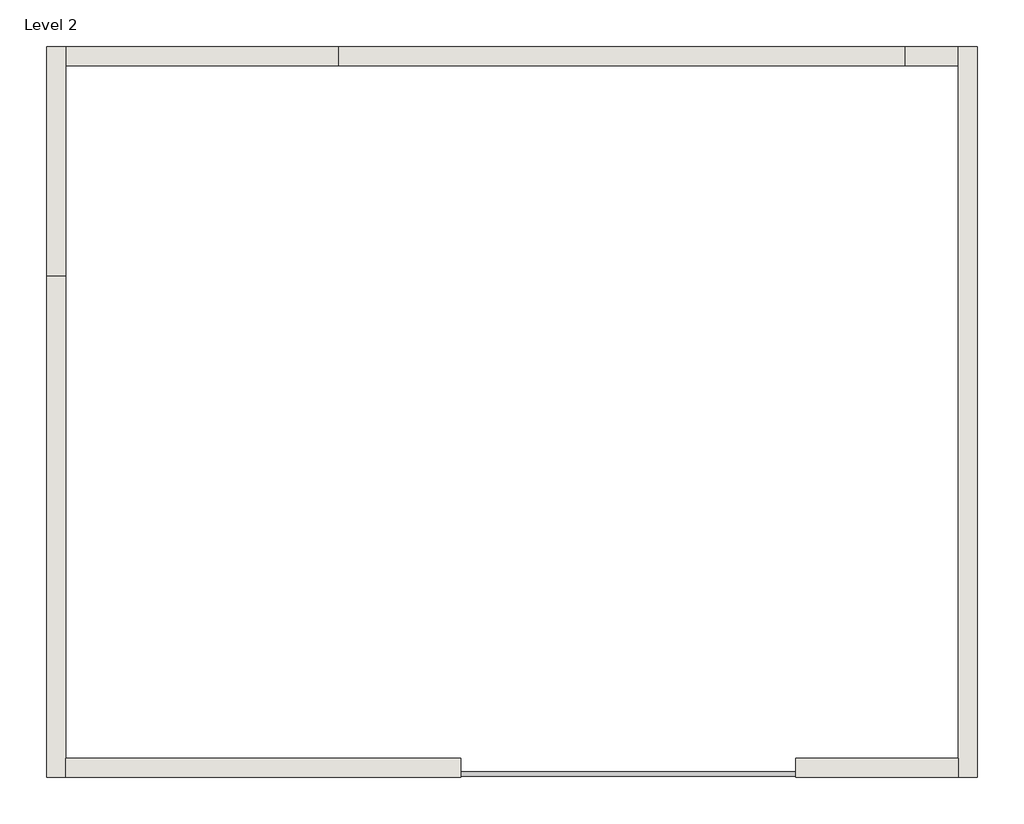
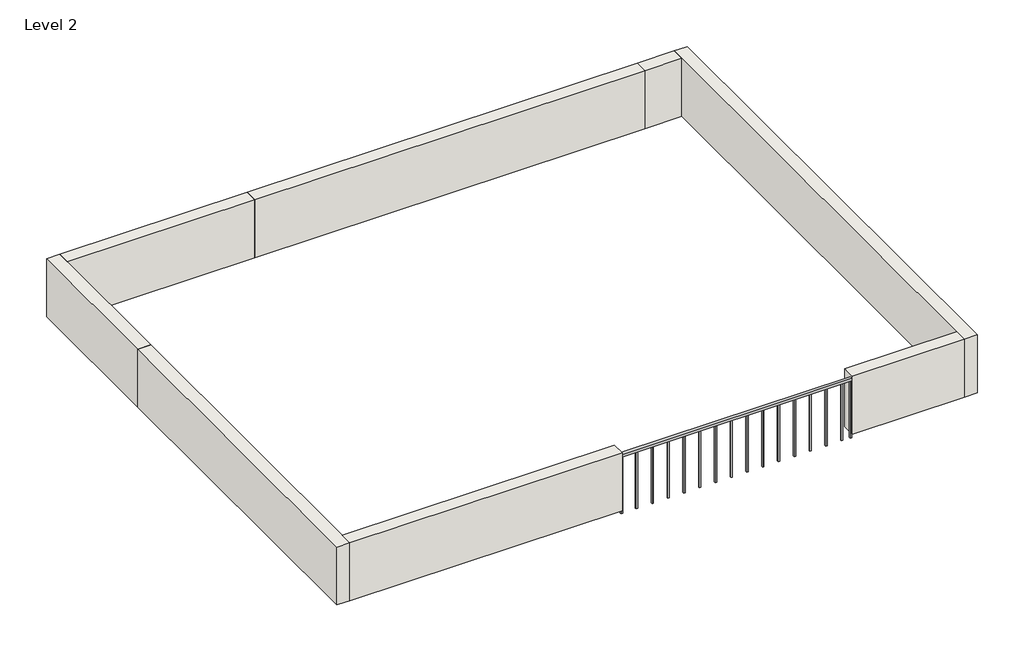
# One storey, incomplete: 8 walls, 1 railing.
"""IFC4 building model written with IfcOpenShell, lengths in millimetres."""

from ifc_helpers import new_model, si_unit, frame, origin, place, context, project, spatial, polyline, outline, extrude, faceted_brep, element, save

model = new_model("IFC4")

# Units and contexts
model_context = context("Model", 3, world=origin())
ifc_project = project(units=[si_unit("LENGTHUNIT", "METRE", prefix="MILLI")], contexts=[model_context])

# Site, building, storey
site = spatial("IfcSite", under=ifc_project)
building = spatial("IfcBuilding", under=site)
storey = spatial("IfcBuildingStorey", under=building, Name="Level 2", Elevation=6400.8)

# Railing
placement = place(None, origin())
element("IfcRailing", 1, ObjectType="1100mm", at=placement, inside=storey, context=model_context, shape_type="SweptSolid", body=[
    extrude(outline(polyline([(-6206.3207599, -3641.6796054), (-6206.3207599, -3591.6796054), (-2193.1207599, -3591.6796054), (-2193.1207599, -3641.6796054), (-6206.3207599, -3641.6796054)])), frame((0.0, 0.0, 7450.8), z_axis=(0.0, 0.0, 1.0), x_axis=(1.0, 0.0, 0.0)), (0.0, 0.0, 1.0), 50.0),
    extrude(outline(polyline([(-2368.8207599, -3629.1796054), (-2368.8207599, -3604.1796054), (-2343.8207599, -3604.1796054), (-2343.8207599, -3629.1796054), (-2368.8207599, -3629.1796054)])), frame((0.0, 0.0, 6400.8), z_axis=(0.0, 0.0, 1.0), x_axis=(1.0, 0.0, 0.0)), (0.0, 0.0, 1.0), 1050.0),
    extrude(outline(polyline([(-2643.8207599, -3629.1796054), (-2643.8207599, -3604.1796054), (-2618.8207599, -3604.1796054), (-2618.8207599, -3629.1796054), (-2643.8207599, -3629.1796054)])), frame((0.0, 0.0, 6400.8), z_axis=(0.0, 0.0, 1.0), x_axis=(1.0, 0.0, 0.0)), (0.0, 0.0, 1.0), 1050.0),
    extrude(outline(polyline([(-2918.8207599, -3629.1796054), (-2918.8207599, -3604.1796054), (-2893.8207599, -3604.1796054), (-2893.8207599, -3629.1796054), (-2918.8207599, -3629.1796054)])), frame((0.0, 0.0, 6400.8), z_axis=(0.0, 0.0, 1.0), x_axis=(1.0, 0.0, 0.0)), (0.0, 0.0, 1.0), 1050.0),
    extrude(outline(polyline([(-3193.8207599, -3629.1796054), (-3193.8207599, -3604.1796054), (-3168.8207599, -3604.1796054), (-3168.8207599, -3629.1796054), (-3193.8207599, -3629.1796054)])), frame((0.0, 0.0, 6400.8), z_axis=(0.0, 0.0, 1.0), x_axis=(1.0, 0.0, 0.0)), (0.0, 0.0, 1.0), 1050.0),
    extrude(outline(polyline([(-3468.8207599, -3629.1796054), (-3468.8207599, -3604.1796054), (-3443.8207599, -3604.1796054), (-3443.8207599, -3629.1796054), (-3468.8207599, -3629.1796054)])), frame((0.0, 0.0, 6400.8), z_axis=(0.0, 0.0, 1.0), x_axis=(1.0, 0.0, 0.0)), (0.0, 0.0, 1.0), 1050.0),
    extrude(outline(polyline([(-3743.8207599, -3629.1796054), (-3743.8207599, -3604.1796054), (-3718.8207599, -3604.1796054), (-3718.8207599, -3629.1796054), (-3743.8207599, -3629.1796054)])), frame((0.0, 0.0, 6400.8), z_axis=(0.0, 0.0, 1.0), x_axis=(1.0, 0.0, 0.0)), (0.0, 0.0, 1.0), 1050.0),
    extrude(outline(polyline([(-4018.8207599, -3629.1796054), (-4018.8207599, -3604.1796054), (-3993.8207599, -3604.1796054), (-3993.8207599, -3629.1796054), (-4018.8207599, -3629.1796054)])), frame((0.0, 0.0, 6400.8), z_axis=(0.0, 0.0, 1.0), x_axis=(1.0, 0.0, 0.0)), (0.0, 0.0, 1.0), 1050.0),
    extrude(outline(polyline([(-4293.8207599, -3629.1796054), (-4293.8207599, -3604.1796054), (-4268.8207599, -3604.1796054), (-4268.8207599, -3629.1796054), (-4293.8207599, -3629.1796054)])), frame((0.0, 0.0, 6400.8), z_axis=(0.0, 0.0, 1.0), x_axis=(1.0, 0.0, 0.0)), (0.0, 0.0, 1.0), 1050.0),
    extrude(outline(polyline([(-4568.8207599, -3629.1796054), (-4568.8207599, -3604.1796054), (-4543.8207599, -3604.1796054), (-4543.8207599, -3629.1796054), (-4568.8207599, -3629.1796054)])), frame((0.0, 0.0, 6400.8), z_axis=(0.0, 0.0, 1.0), x_axis=(1.0, 0.0, 0.0)), (0.0, 0.0, 1.0), 1050.0),
    extrude(outline(polyline([(-4843.8207599, -3629.1796054), (-4843.8207599, -3604.1796054), (-4818.8207599, -3604.1796054), (-4818.8207599, -3629.1796054), (-4843.8207599, -3629.1796054)])), frame((0.0, 0.0, 6400.8), z_axis=(0.0, 0.0, 1.0), x_axis=(1.0, 0.0, 0.0)), (0.0, 0.0, 1.0), 1050.0),
    extrude(outline(polyline([(-5118.8207599, -3629.1796054), (-5118.8207599, -3604.1796054), (-5093.8207599, -3604.1796054), (-5093.8207599, -3629.1796054), (-5118.8207599, -3629.1796054)])), frame((0.0, 0.0, 6400.8), z_axis=(0.0, 0.0, 1.0), x_axis=(1.0, 0.0, 0.0)), (0.0, 0.0, 1.0), 1050.0),
    extrude(outline(polyline([(-5393.8207599, -3629.1796054), (-5393.8207599, -3604.1796054), (-5368.8207599, -3604.1796054), (-5368.8207599, -3629.1796054), (-5393.8207599, -3629.1796054)])), frame((0.0, 0.0, 6400.8), z_axis=(0.0, 0.0, 1.0), x_axis=(1.0, 0.0, 0.0)), (0.0, 0.0, 1.0), 1050.0),
    extrude(outline(polyline([(-5668.8207599, -3629.1796054), (-5668.8207599, -3604.1796054), (-5643.8207599, -3604.1796054), (-5643.8207599, -3629.1796054), (-5668.8207599, -3629.1796054)])), frame((0.0, 0.0, 6400.8), z_axis=(0.0, 0.0, 1.0), x_axis=(1.0, 0.0, 0.0)), (0.0, 0.0, 1.0), 1050.0),
    extrude(outline(polyline([(-5943.8207599, -3629.1796054), (-5943.8207599, -3604.1796054), (-5918.8207599, -3604.1796054), (-5918.8207599, -3629.1796054), (-5943.8207599, -3629.1796054)])), frame((0.0, 0.0, 6400.8), z_axis=(0.0, 0.0, 1.0), x_axis=(1.0, 0.0, 0.0)), (0.0, 0.0, 1.0), 1050.0),
    extrude(outline(polyline([(-2218.1207599, -3629.1796054), (-2218.1207599, -3604.1796054), (-2193.1207599, -3604.1796054), (-2193.1207599, -3629.1796054), (-2218.1207599, -3629.1796054)])), frame((0.0, 0.0, 6400.8), z_axis=(0.0, 0.0, 1.0), x_axis=(1.0, 0.0, 0.0)), (0.0, 0.0, 1.0), 1050.0),
    extrude(outline(polyline([(-6206.3207599, -3629.1796054), (-6206.3207599, -3604.1796054), (-6181.3207599, -3604.1796054), (-6181.3207599, -3629.1796054), (-6206.3207599, -3629.1796054)])), frame((0.0, 0.0, 6400.8), z_axis=(0.0, 0.0, 1.0), x_axis=(1.0, 0.0, 0.0)), (0.0, 0.0, 1.0), 1050.0),
])

# Walls
element("IfcWall", 2, ObjectType="9\"", at=placement, inside=storey, context=model_context, shape_type="Brep", body=[
    faceted_brep([(-13.83523, -3654.7796054, 6477.0), (-13.83523, 5101.6327475, 6477.0), (-13.83523, 5105.4926487, 6477.0), (-13.83523, 5105.4926487, 7543.8), (-13.83523, -3654.7796054, 7543.8), (-242.43523, -3654.7796054, 6477.0), (-242.43523, -3654.7796054, 7543.8), (-242.43523, 4876.8926487, 7543.8), (-242.43523, 5105.4926487, 7543.8), (-242.43523, 5105.4926487, 6477.0), (-242.43523, 4876.8926487, 6477.0)], [[[0, 1, 2, 3, 4]], [[5, 6, 7, 8, 9, 10]], [[2, 1, 0, 5, 10, 9]], [[3, 2, 9, 8]], [[4, 3, 8, 7, 6]], [[0, 4, 6, 5]]]),
])
element("IfcWall", 3, ObjectType="9\"", at=placement, inside=storey, context=model_context, shape_type="SweptSolid", body=[
    extrude(outline(polyline([(-883.78523, 5105.4926487), (-242.43523, 5105.4926487), (-242.43523, 4876.8926487), (-883.78523, 4876.8926487), (-883.78523, 5105.4926487)])), frame((0.0, 0.0, 6477.0), z_axis=(0.0, 0.0, 1.0), x_axis=(1.0, 0.0, 0.0)), (0.0, 0.0, 1.0), 1066.8),
])
element("IfcWall", 4, ObjectType="9\"", at=placement, inside=storey, context=model_context, shape_type="SweptSolid", body=[
    extrude(outline(polyline([(-7680.825513, 5105.4926487), (-883.78523, 5105.4926487), (-883.78523, 4876.8926487), (-7680.825513, 4876.8926487), (-7680.825513, 5105.4926487)])), frame((0.0, 0.0, 6477.0), z_axis=(0.0, 0.0, 1.0), x_axis=(1.0, 0.0, 0.0)), (0.0, 0.0, 1.0), 1066.8),
])
element("IfcWall", 5, ObjectType="9\"", at=placement, inside=storey, context=model_context, shape_type="Brep", body=[
    faceted_brep([(-11175.7858712, 5105.4926487, 6477.0), (-11175.7858712, 2353.0673305, 6477.0), (-11175.7858712, 2353.0673305, 7543.8), (-11175.7858712, 5105.4926487, 7543.8), (-10947.1858712, 5105.4926487, 6477.0), (-10947.1858712, 5105.4926487, 7543.8), (-10947.1858712, 4876.8926487, 7543.8), (-10947.1858712, 2353.0673305, 7543.8), (-10947.1858712, 2353.0673305, 6477.0), (-10947.1858712, 4876.8926487, 6477.0)], [[[0, 1, 2, 3]], [[4, 5, 6, 7, 8, 9]], [[1, 0, 4, 9, 8]], [[2, 1, 8, 7]], [[3, 2, 7, 6, 5]], [[0, 3, 5, 4]]]),
])
element("IfcWall", 6, ObjectType="9\"", at=placement, inside=storey, context=model_context, shape_type="SweptSolid", body=[
    extrude(outline(polyline([(-11175.7858712, -3654.7796054), (-11175.7858712, 2353.0673305), (-10947.1858712, 2353.0673305), (-10947.1858712, -3654.7796054), (-11175.7858712, -3654.7796054)])), frame((0.0, 0.0, 6477.0), z_axis=(0.0, 0.0, 1.0), x_axis=(1.0, 0.0, 0.0)), (0.0, 0.0, 1.0), 1066.8),
])
element("IfcWall", 7, ObjectType="9\"", at=placement, inside=storey, context=model_context, shape_type="SweptSolid", body=[
    extrude(outline(polyline([(-10947.1858712, 5105.4926487), (-7680.825513, 5105.4926487), (-7680.825513, 4876.8926487), (-10947.1858712, 4876.8926487), (-10947.1858712, 5105.4926487)])), frame((0.0, 0.0, 6477.0), z_axis=(0.0, 0.0, 1.0), x_axis=(1.0, 0.0, 0.0)), (0.0, 0.0, 1.0), 1066.8),
])
element("IfcWall", 8, ObjectType="9\"", at=placement, inside=storey, context=model_context, shape_type="SweptSolid", body=[
    extrude(outline(polyline([(-6206.3207599, -3654.7796054), (-10947.1858712, -3654.7796054), (-10947.1858712, -3426.1796054), (-6206.3207599, -3426.1796054), (-6206.3207599, -3654.7796054)])), frame((0.0, 0.0, 6477.0), z_axis=(0.0, 0.0, 1.0), x_axis=(1.0, 0.0, 0.0)), (0.0, 0.0, 1.0), 1066.8),
])
element("IfcWall", 9, ObjectType="9\"", at=placement, inside=storey, context=model_context, shape_type="SweptSolid", body=[
    extrude(outline(polyline([(-242.43523, -3654.7796054), (-2193.1207599, -3654.7796054), (-2193.1207599, -3426.1796054), (-242.43523, -3426.1796054), (-242.43523, -3654.7796054)])), frame((0.0, 0.0, 6477.0), z_axis=(0.0, 0.0, 1.0), x_axis=(1.0, 0.0, 0.0)), (0.0, 0.0, 1.0), 1066.8),
])

save(model, "model.ifc")

# Revit data of these elements
# Type "1100mm"
#   built-in parameter 1008612 = 0.019685 (stored number, unit not read)
#   built-in parameter 1008611 = 0.019685 (stored number, unit not read)
#   built-in parameter 1008609 = 0.902231 (stored number, unit not read)
#   built-in parameter 1008604 = 0.19685 (stored number, unit not read)
#   built-in parameter 1008603 = 0.164042 (stored number, unit not read)
#   Railing Height = 3' - 7.30709"
#   built-in parameter 1008630 = 2
#   built-in parameter 1008610 = 2
#   built-in parameter 1008608 = 1
#   built-in parameter 1008618 = Baluster_Square : 25mm
# Type "9\""
#   Keynote = "F10"
#   Layers, outside or top first: 0' - 9" "Concrete" (function 1)
# Element 1 (IfcRailing, "1100mm")
#   Phase Created = New Construction
# Elements 2, 6 (IfcWall, "9\"")
#   built-in parameter 1001111 = 0' - 3"
#   Top Offset = 0' - 0"
#   Base Offset = 0' - 3"
#   Unconnected Height = 3' - 6"
#   wall height = 3' - 6"
#   Phase Created = New Construction
#   Base Constraint = Level 2
#   Materials on its faces: "Gypsum Wall Board", "Concrete", "Clay Pot"
# Elements 3, 4, 5, 7 (IfcWall, "9\"")
#   built-in parameter 1001111 = 0' - 3"
#   Top Offset = 0' - 0"
#   Base Offset = 0' - 3"
#   Unconnected Height = 3' - 6"
#   wall height = 3' - 6"
#   Phase Created = New Construction
#   Base Constraint = Level 2
#   Materials on its faces: "Gypsum Wall Board", "Concrete"
# Elements 8, 9 (IfcWall, "9\"")
#   built-in parameter 1001111 = 0' - 3"
#   Top Offset = 0' - 0"
#   Base Offset = 0' - 3"
#   Unconnected Height = 3' - 6"
#   wall height = 3' - 6"
#   Phase Created = New Construction
#   Base Constraint = Level 2
#   Materials on its faces: "Concrete", "Gypsum Wall Board", "Clay Pot"
# Materials
#   "Concrete": class "Concrete", colour RGB 120 120 120, transparency 0, Description = "Portland Cement Concrete", Cost = 0
#   "Gypsum Wall Board": class "Generic", colour RGB 249 249 249, transparency 0, Description = "Gypsum Wall Board", Cost = 0
#   "Clay Pot": class "Stucco", colour RGB 237 155 79, transparency 0
